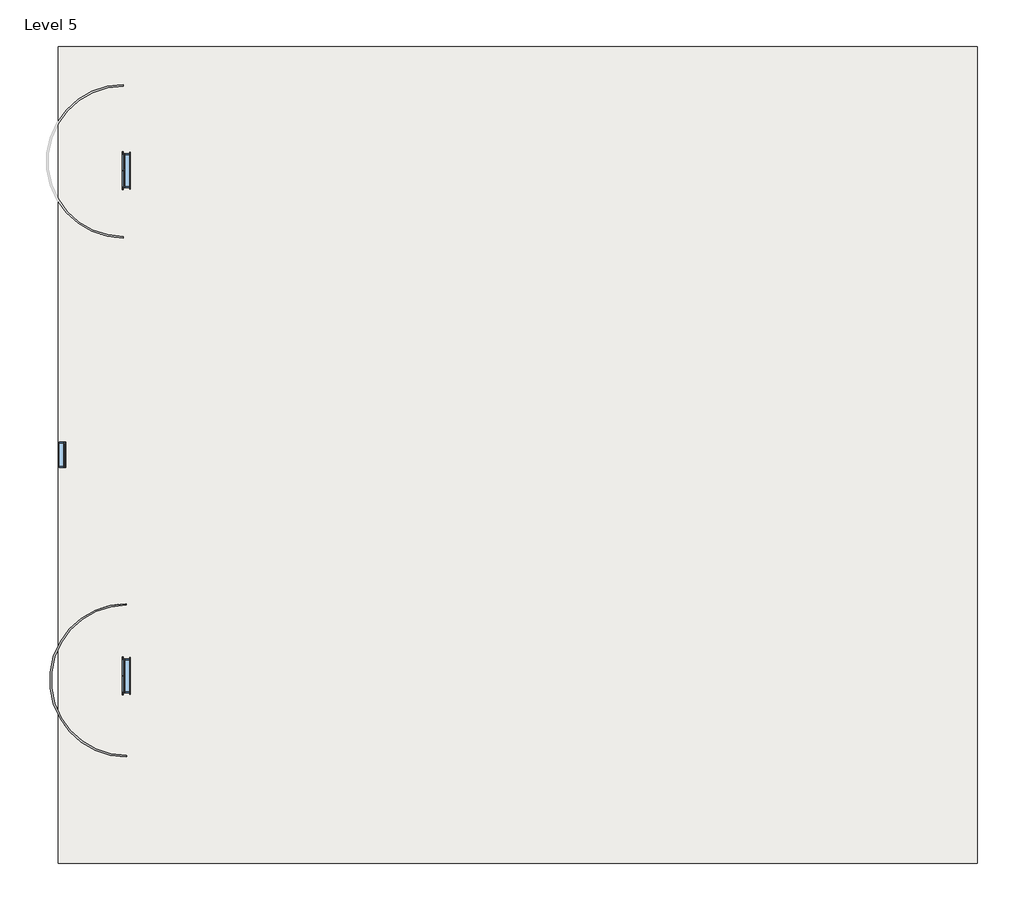
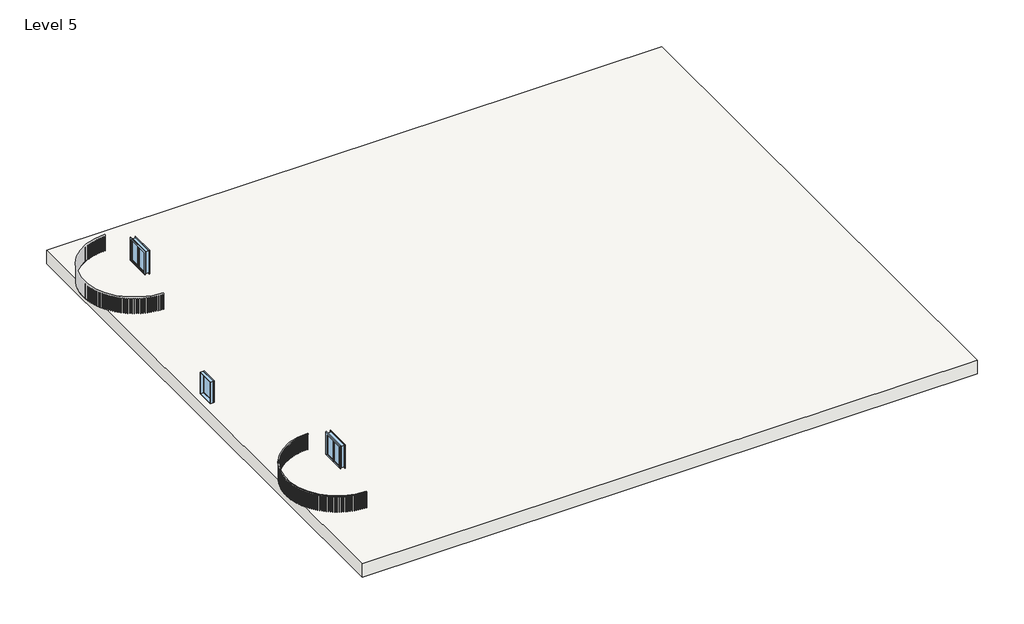
# One storey, part 1 of 2: 3 windows, 1 railing, 1 slab.
"""IFC4 building model written with IfcOpenShell, lengths in millimetres."""

from ifc_helpers import new_model, si_unit, point, frame, frame_2d, origin, place, context, project, spatial, polyline, circle_curve, trimmed, segment, composite_curve, outline, extrude, transform, mapped, element, save
from components import window_534dcd48, window_c1f32544

model = new_model("IFC4")

# Units and contexts
model_context = context("Model", 3, world=origin())
ifc_project = project(units=[si_unit("LENGTHUNIT", "METRE", prefix="MILLI")], contexts=[model_context])

# Site, building, storey
site = spatial("IfcSite", under=ifc_project)
building = spatial("IfcBuilding", under=site)
storey = spatial("IfcBuildingStorey", under=building, Name="Level 5", Elevation=12192.0)

# Railing
placement = place(None, origin())
element("IfcRailing", 1, ObjectType="Handrail - Rectangular", at=placement, inside=storey, context=model_context, shape_type="SweptSolid", body=[
    extrude(outline(composite_curve([segment(trimmed(circle_curve(frame_2d((-15613.8723021, -8267.0443987)), 2743.2), [point((-15613.8723021, -11010.2443987))], [point((-15613.8723021, -5523.8443987))], False, "CARTESIAN"), True, "CONTINUOUS"), segment(polyline([(-15613.8723021, -5523.8443987), (-15613.8723021, -5574.6443987)]), True, "CONTINUOUS"), segment(trimmed(circle_curve(frame_2d((-15613.8723021, -8267.0443987)), 2692.4), [point((-15613.8723021, -5574.6443987))], [point((-15613.8723021, -10959.4443987))], True, "CARTESIAN"), True, "CONTINUOUS"), segment(polyline([(-15613.8723021, -10959.4443987), (-15613.8723021, -11010.2443987)]), True, "CONTINUOUS")], self_intersect=False)), frame((0.0, 0.0, 13055.6), z_axis=(0.0, 0.0, 1.0), x_axis=(1.0, 0.0, 0.0)), (0.0, 0.0, 1.0), 50.8),
    extrude(outline(polyline([(-15627.231195, -10994.3533143), (-15627.2044157, -10975.3033331), (-15608.1544345, -10975.3301124), (-15608.1812138, -10994.3800936), (-15627.231195, -10994.3533143)])), frame((0.0, 0.0, 12192.0), z_axis=(0.0, 0.0, 1.0), x_axis=(1.0, 0.0, 0.0)), (0.0, 0.0, 1.0), 863.6),
    extrude(outline(polyline([(-15729.1535895, -10991.9485449), (-15728.414846, -10972.9128742), (-15709.3791753, -10973.6516178), (-15710.1179188, -10992.6872885), (-15729.1535895, -10991.9485449)])), frame((0.0, 0.0, 12192.0), z_axis=(0.0, 0.0, 1.0), x_axis=(1.0, 0.0, 0.0)), (0.0, 0.0, 1.0), 863.6),
    extrude(outline(polyline([(-15830.914897, -10985.7361601), (-15829.4652214, -10966.7413992), (-15810.4704606, -10968.1910747), (-15811.9201361, -10987.1858356), (-15830.914897, -10985.7361601)])), frame((0.0, 0.0, 12192.0), z_axis=(0.0, 0.0, 1.0), x_axis=(1.0, 0.0, 0.0)), (0.0, 0.0, 1.0), 863.6),
    extrude(outline(polyline([(-15932.3729223, -10975.7248406), (-15930.2143405, -10956.7975316), (-15911.2870315, -10958.9561134), (-15913.4456133, -10977.8834224), (-15932.3729223, -10975.7248406)])), frame((0.0, 0.0, 12192.0), z_axis=(0.0, 0.0, 1.0), x_axis=(1.0, 0.0, 0.0)), (0.0, 0.0, 1.0), 863.6),
    extrude(outline(polyline([(-16033.3858942, -10961.9285757), (-16030.5214224, -10943.0951665), (-16011.6880132, -10945.9596384), (-16014.5524851, -10964.7930475), (-16033.3858942, -10961.9285757)])), frame((0.0, 0.0, 12192.0), z_axis=(0.0, 0.0, 1.0), x_axis=(1.0, 0.0, 0.0)), (0.0, 0.0, 1.0), 863.6),
    extrude(outline(polyline([(-16133.8126634, -10944.3666434), (-16130.2463041, -10925.6534507), (-16111.5331114, -10929.2198099), (-16115.0994706, -10947.9330026), (-16133.8126634, -10944.3666434)])), frame((0.0, 0.0, 12192.0), z_axis=(0.0, 0.0, 1.0), x_axis=(1.0, 0.0, 0.0)), (0.0, 0.0, 1.0), 863.6),
    extrude(outline(polyline([(-16233.5128994, -10923.0635838), (-16229.2496362, -10904.4967562), (-16210.6828086, -10908.7600194), (-16214.9460718, -10927.326847), (-16233.5128994, -10923.0635838)])), frame((0.0, 0.0, 12192.0), z_axis=(0.0, 0.0, 1.0), x_axis=(1.0, 0.0, 0.0)), (0.0, 0.0, 1.0), 863.6),
    extrude(outline(polyline([(-16332.3472874, -10898.0491643), (-16327.3930774, -10879.654646), (-16308.9985591, -10884.608856), (-16313.9527691, -10903.0033743), (-16332.3472874, -10898.0491643)])), frame((0.0, 0.0, 12192.0), z_axis=(0.0, 0.0, 1.0), x_axis=(1.0, 0.0, 0.0)), (0.0, 0.0, 1.0), 863.6),
    extrude(outline(polyline([(-16430.1777221, -10869.3583388), (-16424.5394881, -10851.1618331), (-16406.3429824, -10856.8000671), (-16411.9812164, -10874.9965728), (-16430.1777221, -10869.3583388)])), frame((0.0, 0.0, 12192.0), z_axis=(0.0, 0.0, 1.0), x_axis=(1.0, 0.0, 0.0)), (0.0, 0.0, 1.0), 863.6),
    extrude(outline(polyline([(-16526.8675012, -10837.0311978), (-16520.5531216, -10819.0581316), (-16502.5800554, -10825.3725111), (-16508.8944349, -10843.3455773), (-16526.8675012, -10837.0311978)])), frame((0.0, 0.0, 12192.0), z_axis=(0.0, 0.0, 1.0), x_axis=(1.0, 0.0, 0.0)), (0.0, 0.0, 1.0), 863.6),
    extrude(outline(polyline([(-16622.2815163, -10801.1129136), (-16615.2998146, -10783.3884011), (-16597.5753021, -10790.3701028), (-16604.5570038, -10808.0946153), (-16622.2815163, -10801.1129136)])), frame((0.0, 0.0, 12192.0), z_axis=(0.0, 0.0, 1.0), x_axis=(1.0, 0.0, 0.0)), (0.0, 0.0, 1.0), 863.6),
    extrude(outline(polyline([(-16716.2864416, -10761.653676), (-16708.6471735, -10744.2024845), (-16691.1959821, -10751.8417526), (-16698.8352501, -10769.292944), (-16716.2864416, -10761.653676)])), frame((0.0, 0.0, 12192.0), z_axis=(0.0, 0.0, 1.0), x_axis=(1.0, 0.0, 0.0)), (0.0, 0.0, 1.0), 863.6),
    extrude(outline(polyline([(-16808.7509204, -10718.708623), (-16800.4647607, -10701.5551378), (-16783.3112754, -10709.8412975), (-16791.5974352, -10726.9947828), (-16808.7509204, -10718.708623)])), frame((0.0, 0.0, 12192.0), z_axis=(0.0, 0.0, 1.0), x_axis=(1.0, 0.0, 0.0)), (0.0, 0.0, 1.0), 863.6),
    extrude(outline(polyline([(-16899.5457485, -10672.3377634), (-16890.6242756, -10655.5059536), (-16873.7924658, -10664.4274266), (-16882.7139387, -10681.2592364), (-16899.5457485, -10672.3377634)])), frame((0.0, 0.0, 12192.0), z_axis=(0.0, 0.0, 1.0), x_axis=(1.0, 0.0, 0.0)), (0.0, 0.0, 1.0), 863.6),
    extrude(outline(polyline([(-16988.5440547, -10622.6058931), (-16978.9997349, -10606.1192785), (-16962.5131203, -10615.6635983), (-16972.0574401, -10632.1502129), (-16988.5440547, -10622.6058931)])), frame((0.0, 0.0, 12192.0), z_axis=(0.0, 0.0, 1.0), x_axis=(1.0, 0.0, 0.0)), (0.0, 0.0, 1.0), 863.6),
    extrude(outline(polyline([(-17075.621478, -10569.5825043), (-17065.4676481, -10553.4641223), (-17049.3492661, -10563.6179523), (-17059.5030961, -10579.7363343), (-17075.621478, -10569.5825043)])), frame((0.0, 0.0, 12192.0), z_axis=(0.0, 0.0, 1.0), x_axis=(1.0, 0.0, 0.0)), (0.0, 0.0, 1.0), 863.6),
    extrude(outline(polyline([(-17160.656342, -10513.3416887), (-17149.9071902, -10497.6140622), (-17134.1795637, -10508.363214), (-17144.9287154, -10524.0908405), (-17160.656342, -10513.3416887)])), frame((0.0, 0.0, 12192.0), z_axis=(0.0, 0.0, 1.0), x_axis=(1.0, 0.0, 0.0)), (0.0, 0.0, 1.0), 863.6),
    extrude(outline(polyline([(-17243.5298239, -10453.9620338), (-17232.2003705, -10438.6471396), (-17216.8854763, -10449.976593), (-17228.2149296, -10465.2914872), (-17243.5298239, -10453.9620338)])), frame((0.0, 0.0, 12192.0), z_axis=(0.0, 0.0, 1.0), x_axis=(1.0, 0.0, 0.0)), (0.0, 0.0, 1.0), 863.6),
    extrude(outline(polyline([(-17324.1261214, -10391.5265132), (-17312.2321975, -10376.6457513), (-17297.3514357, -10388.5396752), (-17309.2453596, -10403.4204371), (-17324.1261214, -10391.5265132)])), frame((0.0, 0.0, 12192.0), z_axis=(0.0, 0.0, 1.0), x_axis=(1.0, 0.0, 0.0)), (0.0, 0.0, 1.0), 863.6),
    extrude(outline(polyline([(-17402.3326143, -10326.1223703), (-17389.8908397, -10311.6965343), (-17375.4650036, -10324.1383088), (-17387.9067782, -10338.5641449), (-17402.3326143, -10326.1223703)])), frame((0.0, 0.0, 12192.0), z_axis=(0.0, 0.0, 1.0), x_axis=(1.0, 0.0, 0.0)), (0.0, 0.0, 1.0), 863.6),
    extrude(outline(polyline([(-17478.0400213, -10257.840997), (-17465.0677814, -10243.8902446), (-17451.117029, -10256.8624845), (-17464.0892689, -10270.8132369), (-17478.0400213, -10257.840997)])), frame((0.0, 0.0, 12192.0), z_axis=(0.0, 0.0, 1.0), x_axis=(1.0, 0.0, 0.0)), (0.0, 0.0, 1.0), 863.6),
    extrude(outline(polyline([(-17551.1425537, -10186.7778056), (-17537.6579752, -10173.3216307), (-17524.2018003, -10186.8062093), (-17537.6863789, -10200.2623841), (-17551.1425537, -10186.7778056)])), frame((0.0, 0.0, 12192.0), z_axis=(0.0, 0.0, 1.0), x_axis=(1.0, 0.0, 0.0)), (0.0, 0.0, 1.0), 863.6),
    extrude(outline(polyline([(-17621.5380624, -10113.0320953), (-17607.5599877, -10100.0893009), (-17594.6171933, -10114.0673756), (-17608.595268, -10127.01017), (-17621.5380624, -10113.0320953)])), frame((0.0, 0.0, 12192.0), z_axis=(0.0, 0.0, 1.0), x_axis=(1.0, 0.0, 0.0)), (0.0, 0.0, 1.0), 863.6),
    extrude(outline(polyline([(-17689.128181, -10036.7069141), (-17674.6761422, -10024.2955856), (-17662.2648137, -10038.7476243), (-17676.7168525, -10051.1589528), (-17689.128181, -10036.7069141)])), frame((0.0, 0.0, 12192.0), z_axis=(0.0, 0.0, 1.0), x_axis=(1.0, 0.0, 0.0)), (0.0, 0.0, 1.0), 863.6),
    extrude(outline(polyline([(-17753.8184631, -9957.908914), (-17738.9126547, -9946.0463942), (-17727.0501349, -9960.9522026), (-17741.9559433, -9972.8147224), (-17753.8184631, -9957.908914)])), frame((0.0, 0.0, 12192.0), z_axis=(0.0, 0.0, 1.0), x_axis=(1.0, 0.0, 0.0)), (0.0, 0.0, 1.0), 863.6),
    extrude(outline(polyline([(-17815.5185146, -9876.7482026), (-17800.179765, -9865.4510675), (-17788.8826299, -9880.789817), (-17804.2213795, -9892.0869522), (-17815.5185146, -9876.7482026)])), frame((0.0, 0.0, 12192.0), z_axis=(0.0, 0.0, 1.0), x_axis=(1.0, 0.0, 0.0)), (0.0, 0.0, 1.0), 863.6),
    extrude(outline(polyline([(-17874.1421194, -9793.338189), (-17858.3918621, -9782.6222244), (-17847.6758976, -9798.3724817), (-17863.4261549, -9809.0884462), (-17874.1421194, -9793.338189)])), frame((0.0, 0.0, 12192.0), z_axis=(0.0, 0.0, 1.0), x_axis=(1.0, 0.0, 0.0)), (0.0, 0.0, 1.0), 863.6),
    extrude(outline(polyline([(-17929.6073606, -9707.7954251), (-17913.467604, -9697.6756051), (-17903.347784, -9713.8153616), (-17919.4875405, -9723.9351817), (-17929.6073606, -9707.7954251)])), frame((0.0, 0.0, 12192.0), z_axis=(0.0, 0.0, 1.0), x_axis=(1.0, 0.0, 0.0)), (0.0, 0.0, 1.0), 863.6),
    extrude(outline(polyline([(-17981.8367343, -9620.2394434), (-17965.3300312, -9610.7299086), (-17955.8204964, -9627.2366117), (-17972.3271995, -9636.7461465), (-17981.8367343, -9620.2394434)])), frame((0.0, 0.0, 12192.0), z_axis=(0.0, 0.0, 1.0), x_axis=(1.0, 0.0, 0.0)), (0.0, 0.0, 1.0), 863.6),
    extrude(outline(polyline([(-18030.7572585, -9530.7925891), (-18013.9066743, -9521.9066277), (-18005.0207128, -9538.7572119), (-18021.871297, -9547.6431733), (-18030.7572585, -9530.7925891)])), frame((0.0, 0.0, 12192.0), z_axis=(0.0, 0.0, 1.0), x_axis=(1.0, 0.0, 0.0)), (0.0, 0.0, 1.0), 863.6),
    extrude(outline(polyline([(-18076.3005745, -9439.5798499), (-18059.1296552, -9431.3298785), (-18050.8796837, -9448.5007978), (-18068.0506031, -9456.7507693), (-18076.3005745, -9439.5798499)])), frame((0.0, 0.0, 12192.0), z_axis=(0.0, 0.0, 1.0), x_axis=(1.0, 0.0, 0.0)), (0.0, 0.0, 1.0), 863.6),
    extrude(outline(polyline([(-18118.4030429, -9346.728681), (-18100.9357821, -9339.1262276), (-18093.3333287, -9356.5934885), (-18110.8005895, -9364.1959419), (-18118.4030429, -9346.728681)])), frame((0.0, 0.0, 12192.0), z_axis=(0.0, 0.0, 1.0), x_axis=(1.0, 0.0, 0.0)), (0.0, 0.0, 1.0), 863.6),
    extrude(outline(polyline([(-18157.0058323, -9252.3688268), (-18139.2666376, -9245.4245147), (-18132.3223254, -9263.1637094), (-18150.0615201, -9270.1080215), (-18157.0058323, -9252.3688268)])), frame((0.0, 0.0, 12192.0), z_axis=(0.0, 0.0, 1.0), x_axis=(1.0, 0.0, 0.0)), (0.0, 0.0, 1.0), 863.6),
    extrude(outline(polyline([(-18192.0550015, -9156.6321402), (-18174.0686606, -9150.3556729), (-18167.7921932, -9168.3420137), (-18185.7785341, -9174.6184811), (-18192.0550015, -9156.6321402)])), frame((0.0, 0.0, 12192.0), z_axis=(0.0, 0.0, 1.0), x_axis=(1.0, 0.0, 0.0)), (0.0, 0.0, 1.0), 863.6),
    extrude(outline(polyline([(-18223.5015748, -9059.6523978), (-18205.2932208, -9054.0525456), (-18199.6933686, -9072.2608996), (-18217.9017226, -9077.8607518), (-18223.5015748, -9059.6523978)])), frame((0.0, 0.0, 12192.0), z_axis=(0.0, 0.0, 1.0), x_axis=(1.0, 0.0, 0.0)), (0.0, 0.0, 1.0), 863.6),
    extrude(outline(polyline([(-18251.3016108, -8961.5651131), (-18232.8966869, -8956.6497009), (-18227.9812748, -8975.0546248), (-18246.3861986, -8979.970037), (-18251.3016108, -8961.5651131)])), frame((0.0, 0.0, 12192.0), z_axis=(0.0, 0.0, 1.0), x_axis=(1.0, 0.0, 0.0)), (0.0, 0.0, 1.0), 863.6),
    extrude(outline(polyline([(-18275.4162634, -8862.5073473), (-18256.8404876, -8858.2832437), (-18252.6163839, -8876.8590196), (-18271.1921598, -8881.0831232), (-18275.4162634, -8862.5073473)])), frame((0.0, 0.0, 12192.0), z_axis=(0.0, 0.0, 1.0), x_axis=(1.0, 0.0, 0.0)), (0.0, 0.0, 1.0), 863.6),
    extrude(outline(polyline([(-18295.8118362, -8762.6175179), (-18277.0911651, -8759.0906253), (-18273.5642725, -8777.8112965), (-18292.2849436, -8781.338189), (-18295.8118362, -8762.6175179)])), frame((0.0, 0.0, 12192.0), z_axis=(0.0, 0.0, 1.0), x_axis=(1.0, 0.0, 0.0)), (0.0, 0.0, 1.0), 863.6),
    extrude(outline(polyline([(-18312.4598298, -8662.0352047), (-18293.6204224, -8659.2104514), (-18290.7956691, -8678.0498587), (-18309.6350765, -8680.874612), (-18312.4598298, -8662.0352047)])), frame((0.0, 0.0, 12192.0), z_axis=(0.0, 0.0, 1.0), x_axis=(1.0, 0.0, 0.0)), (0.0, 0.0, 1.0), 863.6),
    extrude(outline(polyline([(-18325.3369811, -8560.9009553), (-18306.4051626, -8558.7822885), (-18304.2864958, -8577.714107), (-18323.2183143, -8579.8327738), (-18325.3369811, -8560.9009553)])), frame((0.0, 0.0, 12192.0), z_axis=(0.0, 0.0, 1.0), x_axis=(1.0, 0.0, 0.0)), (0.0, 0.0, 1.0), 863.6),
    extrude(outline(polyline([(-18334.4252965, -8459.3560886), (-18315.427521, -8457.9464688), (-18314.0179011, -8476.9442442), (-18333.0156766, -8478.3538641), (-18334.4252965, -8459.3560886)])), frame((0.0, 0.0, 12192.0), z_axis=(0.0, 0.0, 1.0), x_axis=(1.0, 0.0, 0.0)), (0.0, 0.0, 1.0), 863.6),
    extrude(outline(polyline([(-18339.7120764, -8357.5424973), (-18320.6748904, -8356.8438941), (-18319.9762872, -8375.8810802), (-18339.0134732, -8376.5796834), (-18339.7120764, -8357.5424973)])), frame((0.0, 0.0, 12192.0), z_axis=(0.0, 0.0, 1.0), x_axis=(1.0, 0.0, 0.0)), (0.0, 0.0, 1.0), 863.6),
    extrude(outline(polyline([(-18341.1899336, -8255.6024494), (-18322.1399383, -8255.6158391), (-18322.1533279, -8274.6658344), (-18341.2033232, -8274.6524447), (-18341.1899336, -8255.6024494)])), frame((0.0, 0.0, 12192.0), z_axis=(0.0, 0.0, 1.0), x_axis=(1.0, 0.0, 0.0)), (0.0, 0.0, 1.0), 863.6),
    extrude(outline(polyline([(-18338.8568028, -8153.6783898), (-18319.8206176, -8154.4037536), (-18320.5459814, -8173.4399388), (-18339.5821666, -8172.7145751), (-18338.8568028, -8153.6783898)])), frame((0.0, 0.0, 12192.0), z_axis=(0.0, 0.0, 1.0), x_axis=(1.0, 0.0, 0.0)), (0.0, 0.0, 1.0), 863.6),
    extrude(outline(polyline([(-18332.7159444, -8051.912741), (-18313.7201692, -8053.3490654), (-18315.1564936, -8072.3448405), (-18334.1522687, -8070.9085161), (-18332.7159444, -8051.912741)])), frame((0.0, 0.0, 12192.0), z_axis=(0.0, 0.0, 1.0), x_axis=(1.0, 0.0, 0.0)), (0.0, 0.0, 1.0), 863.6),
    extrude(outline(polyline([(-18322.775939, -7950.4477041), (-18303.8471175, -7952.592982), (-18305.9923954, -7971.5218035), (-18324.9212169, -7969.3765256), (-18322.775939, -7950.4477041)])), frame((0.0, 0.0, 12192.0), z_axis=(0.0, 0.0, 1.0), x_axis=(1.0, 0.0, 0.0)), (0.0, 0.0, 1.0), 863.6),
    extrude(outline(polyline([(-18309.0506764, -7849.4250602), (-18290.2152585, -7852.2762939), (-18293.0664923, -7871.1117118), (-18311.9019101, -7868.260478), (-18309.0506764, -7849.4250602)])), frame((0.0, 0.0, 12192.0), z_axis=(0.0, 0.0, 1.0), x_axis=(1.0, 0.0, 0.0)), (0.0, 0.0, 1.0), 863.6),
    extrude(outline(polyline([(-18291.5593353, -7748.9859721), (-18272.8436405, -7752.5391776), (-18276.396846, -7771.2548723), (-18295.1125408, -7767.7016669), (-18291.5593353, -7748.9859721)])), frame((0.0, 0.0, 12192.0), z_axis=(0.0, 0.0, 1.0), x_axis=(1.0, 0.0, 0.0)), (0.0, 0.0, 1.0), 863.6),
    extrude(outline(polyline([(-18270.3263571, -7649.2707874), (-18251.7565376, -7653.5209995), (-18256.0067497, -7672.0908191), (-18274.5765692, -7667.8406069), (-18270.3263571, -7649.2707874)])), frame((0.0, 0.0, 12192.0), z_axis=(0.0, 0.0, 1.0), x_axis=(1.0, 0.0, 0.0)), (0.0, 0.0, 1.0), 863.6),
    extrude(outline(polyline([(-18245.3814115, -7550.418842), (-18226.9834156, -7555.3601218), (-18231.9246954, -7573.7581178), (-18250.3226913, -7568.816838), (-18245.3814115, -7550.418842)])), frame((0.0, 0.0, 12192.0), z_axis=(0.0, 0.0, 1.0), x_axis=(1.0, 0.0, 0.0)), (0.0, 0.0, 1.0), 863.6),
    extrude(outline(polyline([(-18216.7593549, -7452.5682656), (-18198.5588909, -7458.1937085), (-18204.1843337, -7476.3941726), (-18222.3847978, -7470.7687297), (-18216.7593549, -7452.5682656)])), frame((0.0, 0.0, 12192.0), z_axis=(0.0, 0.0, 1.0), x_axis=(1.0, 0.0, 0.0)), (0.0, 0.0, 1.0), 863.6),
    extrude(outline(polyline([(-18184.5001822, -7355.8557887), (-18166.5226822, -7362.1575339), (-18172.8244275, -7380.1350339), (-18190.8019275, -7373.8332887), (-18184.5001822, -7355.8557887)])), frame((0.0, 0.0, 12192.0), z_axis=(0.0, 0.0, 1.0), x_axis=(1.0, 0.0, 0.0)), (0.0, 0.0, 1.0), 863.6),
    extrude(outline(polyline([(-18148.6489704, -7260.4165513), (-18130.9195551, -7267.3857933), (-18137.888797, -7285.1152086), (-18155.6182123, -7278.1459666), (-18148.6489704, -7260.4165513)])), frame((0.0, 0.0, 12192.0), z_axis=(0.0, 0.0, 1.0), x_axis=(1.0, 0.0, 0.0)), (0.0, 0.0, 1.0), 863.6),
    extrude(outline(polyline([(-18109.2558157, -7166.3839145), (-18091.7992591, -7174.0109148), (-18099.4262594, -7191.4674713), (-18116.8828159, -7183.8404711), (-18109.2558157, -7166.3839145)])), frame((0.0, 0.0, 12192.0), z_axis=(0.0, 0.0, 1.0), x_axis=(1.0, 0.0, 0.0)), (0.0, 0.0, 1.0), 863.6),
    extrude(outline(polyline([(-18066.3757637, -7073.8892738), (-18049.2164586, -7082.1633749), (-18057.4905597, -7099.32268), (-18074.6498648, -7091.0485789), (-18066.3757637, -7073.8892738)])), frame((0.0, 0.0, 12192.0), z_axis=(0.0, 0.0, 1.0), x_axis=(1.0, 0.0, 0.0)), (0.0, 0.0, 1.0), 863.6),
    extrude(outline(polyline([(-18020.0687324, -6983.0618755), (-18003.2306562, -6991.9715157), (-18012.1402963, -7008.8095919), (-18028.9783726, -6999.8999518), (-18020.0687324, -6983.0618755)])), frame((0.0, 0.0, 12192.0), z_axis=(0.0, 0.0, 1.0), x_axis=(1.0, 0.0, 0.0)), (0.0, 0.0, 1.0), 863.6),
    extrude(outline(polyline([(-17970.3994285, -6894.0286364), (-17953.9061096, -6903.5613658), (-17963.4388391, -6920.0546848), (-17979.932158, -6910.5219553), (-17970.3994285, -6894.0286364)])), frame((0.0, 0.0, 12192.0), z_axis=(0.0, 0.0, 1.0), x_axis=(1.0, 0.0, 0.0)), (0.0, 0.0, 1.0), 863.6),
    extrude(outline(polyline([(-17917.4372568, -6806.913966), (-17901.311742, -6817.0564643), (-17911.4542403, -6833.1819791), (-17927.5797552, -6823.0394808), (-17917.4372568, -6806.913966)])), frame((0.0, 0.0, 12192.0), z_axis=(0.0, 0.0, 1.0), x_axis=(1.0, 0.0, 0.0)), (0.0, 0.0, 1.0), 863.6),
    extrude(outline(polyline([(-17861.2562235, -6721.8395932), (-17845.5210456, -6732.5776878), (-17856.2591402, -6748.3128657), (-17871.9943181, -6737.5747711), (-17861.2562235, -6721.8395932)])), frame((0.0, 0.0, 12192.0), z_axis=(0.0, 0.0, 1.0), x_axis=(1.0, 0.0, 0.0)), (0.0, 0.0, 1.0), 863.6),
    extrude(outline(polyline([(-17801.9348324, -6638.9243956), (-17786.6119788, -6650.2430818), (-17797.9306651, -6665.5659354), (-17813.2535187, -6654.2472492), (-17801.9348324, -6638.9243956)])), frame((0.0, 0.0, 12192.0), z_axis=(0.0, 0.0, 1.0), x_axis=(1.0, 0.0, 0.0)), (0.0, 0.0, 1.0), 863.6),
    extrude(outline(polyline([(-17739.5559758, -6558.284234), (-17724.6668577, -6570.1676957), (-17736.5503195, -6585.0568138), (-17751.4394375, -6573.1733521), (-17739.5559758, -6558.284234)])), frame((0.0, 0.0, 12192.0), z_axis=(0.0, 0.0, 1.0), x_axis=(1.0, 0.0, 0.0)), (0.0, 0.0, 1.0), 863.6),
    extrude(outline(polyline([(-17674.206818, -6480.03179), (-17659.7722406, -6492.463422), (-17672.2038726, -6506.8979994), (-17686.63845, -6494.4663674), (-17674.206818, -6480.03179)])), frame((0.0, 0.0, 12192.0), z_axis=(0.0, 0.0, 1.0), x_axis=(1.0, 0.0, 0.0)), (0.0, 0.0, 1.0), 863.6),
    extrude(outline(polyline([(-17605.978674, -6404.2764087), (-17592.0188072, -6417.2388399), (-17604.9812384, -6431.1987066), (-17618.9411051, -6418.2362755), (-17605.978674, -6404.2764087)])), frame((0.0, 0.0, 12192.0), z_axis=(0.0, 0.0, 1.0), x_axis=(1.0, 0.0, 0.0)), (0.0, 0.0, 1.0), 863.6),
    extrude(outline(polyline([(-17534.9668816, -6331.1239463), (-17521.5012322, -6344.5990636), (-17534.9763495, -6358.064713), (-17548.4419989, -6344.5895957), (-17534.9668816, -6331.1239463)])), frame((0.0, 0.0, 12192.0), z_axis=(0.0, 0.0, 1.0), x_axis=(1.0, 0.0, 0.0)), (0.0, 0.0, 1.0), 863.6),
    extrude(outline(polyline([(-17461.2706683, -6260.6766214), (-17448.3180524, -6274.6455956), (-17462.2870265, -6287.5982116), (-17475.2396425, -6273.6292374), (-17461.2706683, -6260.6766214)])), frame((0.0, 0.0, 12192.0), z_axis=(0.0, 0.0, 1.0), x_axis=(1.0, 0.0, 0.0)), (0.0, 0.0, 1.0), 863.6),
    extrude(outline(polyline([(-17384.9930129, -6193.032873), (-17372.5715296, -6207.4761846), (-17387.0148412, -6219.897668), (-17399.4363246, -6205.4543563), (-17384.9930129, -6193.032873)])), frame((0.0, 0.0, 12192.0), z_axis=(0.0, 0.0, 1.0), x_axis=(1.0, 0.0, 0.0)), (0.0, 0.0, 1.0), 863.6),
    extrude(outline(polyline([(-17306.2405011, -6128.2872222), (-17294.3675074, -6143.1846891), (-17309.2649743, -6155.0576828), (-17321.137968, -6140.1602159), (-17306.2405011, -6128.2872222)])), frame((0.0, 0.0, 12192.0), z_axis=(0.0, 0.0, 1.0), x_axis=(1.0, 0.0, 0.0)), (0.0, 0.0, 1.0), 863.6),
    extrude(outline(polyline([(-17225.1231768, -6066.5301406), (-17213.8152633, -6081.860946), (-17229.1460687, -6093.1688594), (-17240.4539822, -6077.8380541), (-17225.1231768, -6066.5301406)])), frame((0.0, 0.0, 12192.0), z_axis=(0.0, 0.0, 1.0), x_axis=(1.0, 0.0, 0.0)), (0.0, 0.0, 1.0), 863.6),
    extrude(outline(polyline([(-17141.7543884, -6007.847924), (-17131.0273562, -6023.5906455), (-17146.7700777, -6034.3176777), (-17157.4971099, -6018.5749562), (-17141.7543884, -6007.847924)])), frame((0.0, 0.0, 12192.0), z_axis=(0.0, 0.0, 1.0), x_axis=(1.0, 0.0, 0.0)), (0.0, 0.0, 1.0), 863.6),
    extrude(outline(polyline([(-17056.2506305, -5952.3225712), (-17046.1194688, -5968.4552108), (-17062.2521085, -5978.5863725), (-17072.3832702, -5962.4537328), (-17056.2506305, -5952.3225712)])), frame((0.0, 0.0, 12192.0), z_axis=(0.0, 0.0, 1.0), x_axis=(1.0, 0.0, 0.0)), (0.0, 0.0, 1.0), 863.6),
    extrude(outline(polyline([(-16968.7313808, -5900.03167), (-16959.2102463, -5916.5316851), (-16975.7102614, -5926.0528195), (-16985.2313959, -5909.5528044), (-16968.7313808, -5900.03167)])), frame((0.0, 0.0, 12192.0), z_axis=(0.0, 0.0, 1.0), x_axis=(1.0, 0.0, 0.0)), (0.0, 0.0, 1.0), 863.6),
    extrude(outline(polyline([(-16879.3189333, -5851.0482885), (-16870.4211303, -5867.8926229), (-16887.2654647, -5876.7904259), (-16896.1632677, -5859.9460915), (-16879.3189333, -5851.0482885)])), frame((0.0, 0.0, 12192.0), z_axis=(0.0, 0.0, 1.0), x_axis=(1.0, 0.0, 0.0)), (0.0, 0.0, 1.0), 863.6),
    extrude(outline(polyline([(-16788.1382277, -5805.4408731), (-16779.8761894, -5822.6059896), (-16797.0413058, -5830.8680279), (-16805.3033441, -5813.7029114), (-16788.1382277, -5805.4408731)])), frame((0.0, 0.0, 12192.0), z_axis=(0.0, 0.0, 1.0), x_axis=(1.0, 0.0, 0.0)), (0.0, 0.0, 1.0), 863.6),
    extrude(outline(polyline([(-16695.3166742, -5763.2731529), (-16687.7019455, -5780.7350659), (-16705.1638585, -5788.3497946), (-16712.7785872, -5770.8878816), (-16695.3166742, -5763.2731529)])), frame((0.0, 0.0, 12192.0), z_axis=(0.0, 0.0, 1.0), x_axis=(1.0, 0.0, 0.0)), (0.0, 0.0, 1.0), 863.6),
    extrude(outline(polyline([(-16600.983976, -5724.6040505), (-16594.0271973, -5742.3383598), (-16611.7615066, -5749.2951386), (-16618.7182854, -5731.5608292), (-16600.983976, -5724.6040505)])), frame((0.0, 0.0, 12192.0), z_axis=(0.0, 0.0, 1.0), x_axis=(1.0, 0.0, 0.0)), (0.0, 0.0, 1.0), 863.6),
    extrude(outline(polyline([(-16505.271948, -5689.4875996), (-16498.9828402, -5707.4695245), (-16516.9647651, -5713.7586324), (-16523.2538729, -5695.7767075), (-16505.271948, -5689.4875996)])), frame((0.0, 0.0, 12192.0), z_axis=(0.0, 0.0, 1.0), x_axis=(1.0, 0.0, 0.0)), (0.0, 0.0, 1.0), 863.6),
    extrude(outline(polyline([(-16408.3143324, -5657.97287), (-16402.7016834, -5676.1772836), (-16420.906097, -5681.7899325), (-16426.5187459, -5663.5855189), (-16408.3143324, -5657.97287)])), frame((0.0, 0.0, 12192.0), z_axis=(0.0, 0.0, 1.0), x_axis=(1.0, 0.0, 0.0)), (0.0, 0.0, 1.0), 863.6),
    extrude(outline(polyline([(-16310.2466117, -5630.1038984), (-16305.3182645, -5648.5053628), (-16323.7197289, -5653.43371), (-16328.6480761, -5635.0322456), (-16310.2466117, -5630.1038984)])), frame((0.0, 0.0, 12192.0), z_axis=(0.0, 0.0, 1.0), x_axis=(1.0, 0.0, 0.0)), (0.0, 0.0, 1.0), 863.6),
    extrude(outline(polyline([(-16211.2058198, -5605.9196271), (-16206.9686609, -5624.4924294), (-16225.5414632, -5628.7295883), (-16229.7786221, -5610.1567861), (-16211.2058198, -5605.9196271)])), frame((0.0, 0.0, 12192.0), z_axis=(0.0, 0.0, 1.0), x_axis=(1.0, 0.0, 0.0)), (0.0, 0.0, 1.0), 863.6),
    extrude(outline(polyline([(-16111.3303505, -5585.4538499), (-16107.7903006, -5604.1720375), (-16126.5084882, -5607.7120874), (-16130.048538, -5588.9938998), (-16111.3303505, -5585.4538499)])), frame((0.0, 0.0, 12192.0), z_axis=(0.0, 0.0, 1.0), x_axis=(1.0, 0.0, 0.0)), (0.0, 0.0, 1.0), 863.6),
    extrude(outline(polyline([(-16010.7597634, -5568.7351643), (-16007.9217692, -5587.5725816), (-16026.7591865, -5590.4105758), (-16029.5971807, -5571.5731585), (-16010.7597634, -5568.7351643)])), frame((0.0, 0.0, 12192.0), z_axis=(0.0, 0.0, 1.0), x_axis=(1.0, 0.0, 0.0)), (0.0, 0.0, 1.0), 863.6),
    extrude(outline(polyline([(-15909.63459, -5555.7869321), (-15907.5026171, -5574.7172567), (-15926.4329418, -5576.8492296), (-15928.5649146, -5557.918905), (-15909.63459, -5555.7869321)])), frame((0.0, 0.0, 12192.0), z_axis=(0.0, 0.0, 1.0), x_axis=(1.0, 0.0, 0.0)), (0.0, 0.0, 1.0), 863.6),
    extrude(outline(polyline([(-15808.0961363, -5546.6272462), (-15806.6731638, -5565.6240262), (-15825.6699438, -5567.0469987), (-15827.0929163, -5548.0502187), (-15808.0961363, -5546.6272462)])), frame((0.0, 0.0, 12192.0), z_axis=(0.0, 0.0, 1.0), x_axis=(1.0, 0.0, 0.0)), (0.0, 0.0, 1.0), 863.6),
    extrude(outline(polyline([(-15706.286286, -5541.268906), (-15705.5743024, -5560.3055963), (-15724.6109927, -5561.01758), (-15725.3229764, -5541.9808896), (-15706.286286, -5541.268906)])), frame((0.0, 0.0, 12192.0), z_axis=(0.0, 0.0, 1.0), x_axis=(1.0, 0.0, 0.0)), (0.0, 0.0, 1.0), 863.6),
    extrude(outline(polyline([(-15632.955606, -10994.3192673), (-15632.8888422, -10975.2693843), (-15613.8389591, -10975.3361482), (-15613.905723, -10994.3860312), (-15632.955606, -10994.3192673)])), frame((0.0, 0.0, 12192.0), z_axis=(0.0, 0.0, 1.0), x_axis=(1.0, 0.0, 0.0)), (0.0, 0.0, 1.0), 863.6),
    extrude(outline(polyline([(-15613.905723, -5539.7027662), (-15613.8389591, -5558.7526493), (-15632.8888422, -5558.8194131), (-15632.955606, -5539.7695301), (-15613.905723, -5539.7027662)])), frame((0.0, 0.0, 12192.0), z_axis=(0.0, 0.0, 1.0), x_axis=(1.0, 0.0, 0.0)), (0.0, 0.0, 1.0), 863.6),
])

# Slab
element("IfcSlab", 2, ObjectType="Generic - 12\"", at=placement, inside=storey, context=model_context, shape_type="SweptSolid", body=[
    extrude(outline(polyline([(14866.1276979, 14440.5556013), (14866.1276979, -14820.2443987), (-18052.2723021, -14820.2443987), (-18052.2723021, 14440.5556013), (14866.1276979, 14440.5556013)])), frame((0.0, 0.0, 11430.0), z_axis=(0.0, 0.0, 1.0), x_axis=(1.0, 0.0, 0.0)), (0.0, 0.0, 1.0), 762.0),
])

# Windows
window_shape = window_534dcd48(model_context)
element("IfcWindow", 3, ObjectType="Casement Dbl with Trim : 48\" x 48\"", at=placement, inside=storey, context=model_context, shape_type="MappedRepresentation", body=[
    mapped(window_shape, transform((-15594.8223021, 9995.5556013, 12192.0), x_axis=(0.0, 1.0, 0.0), y_axis=(-1.0, 0.0, 0.0), z_axis=(0.0, 0.0, 1.0))),
])
element("IfcWindow", 4, ObjectType="Casement Dbl with Trim : 48\" x 48\"", at=placement, inside=storey, context=model_context, shape_type="MappedRepresentation", body=[
    mapped(window_shape, transform((-15594.8223021, -8114.6443987, 12192.0), x_axis=(0.0, 1.0, 0.0), y_axis=(-1.0, 0.0, 0.0), z_axis=(0.0, 0.0, 1.0))),
])
window_2_shape = window_c1f32544(model_context)
element("IfcWindow", 5, ObjectType="Fixed : 36\" x 48\"", at=placement, inside=storey, context=model_context, shape_type="MappedRepresentation", body=[
    mapped(window_2_shape, transform((-17899.8723021, -227.9443987, 11735.1091362), x_axis=(0.0, -1.0, 0.0), y_axis=(1.0, 0.0, 0.0), z_axis=(0.0, 0.0, 1.0))),
])

save(model, "model.ifc")

# Revit data of these elements
# Type "Handrail - Rectangular"
#   Assembly Code = "C2010400"
#   built-in parameter 1008612 = 0.0416667 (stored number, unit not read)
#   built-in parameter 1008611 = 0.0416667 (stored number, unit not read)
#   built-in parameter 1008609 = 0.333333 (stored number, unit not read)
#   built-in parameter 1008604 = 0.166667 (stored number, unit not read)
#   built-in parameter 1008603 = 0.166667 (stored number, unit not read)
#   Railing Height = 3' - 0"
#   built-in parameter 1008630 = 2
#   built-in parameter 1008610 = 2
#   built-in parameter 1008618 = Baluster - Square : 3/4"
# Type "Generic - 12\""
#   Assembly Code = "B1010"
#   Function = 0
#   Layers, outside or top first: 2' - 6" no material (function 1)
# Type "Casement Dbl with Trim : 48\" x 48\""
#   Type Mark = "19"
#   Construction Type Id = "GSP4R"
#   Assembly Code = "B2020100"
#   Analytic Construction = "1/8 in Pilkington single glazing"
#   Visual Light Transmittance = 0.9
#   Solar Heat Gain Coefficient = 0.78
#   Heat Transfer Coefficient (U) = 0.6496 BTU/(h·ft²·°F)
#   Height = 4' - 0"
#   Default Sill Height = 3' - 0"
#   Trim Projection - Ext. = 0' - 0 1/2"
#   Trim Projection - Int. = 0' - 0 3/4"
#   Trim Width - Exterior = 0' - 3 1/2"
#   Trim Width - Interior = 0' - 3 1/2"
#   Width = 4' - 0"
#   Window Inset = 0' - 0 3/4"
#   Define Thermal Properties by = 1
#   Glass Pane Material = Glass
#   Sash Material = Sash
#   Trim Exterior Material = Trim
#   Trim Interior Material = Trim
#   Wall Closure = (empty or 0)
# Type "Fixed : 36\" x 48\""
#   Type Mark = "1"
#   Construction Type Id = "GSP4R"
#   Assembly Code = "B2020100"
#   Analytic Construction = "1/8 in Pilkington single glazing"
#   Visual Light Transmittance = 0.9
#   Solar Heat Gain Coefficient = 0.78
#   Heat Transfer Coefficient (U) = 0.6496 BTU/(h·ft²·°F)
#   Height = 4' - 0"
#   Default Sill Height = 3' - 0"
#   Width = 3' - 0"
#   Window Inset = 0' - 0 3/4"
#   Define Thermal Properties by = 1
#   Glass Pane Material = Glass
#   Sash Material = Sash
#   Wall Closure = (empty or 0)
# Element 1 (IfcRailing, "Handrail - Rectangular")
#   Phase Created = New Construction
# Element 2 (IfcSlab, "Generic - 12\"")
#   Height Offset From Level = 0' - 0"
#   Phase Created = New Construction
#   Materials on its faces: "Default Floor"
# Element 3 (IfcWindow, "Casement Dbl with Trim : 48\" x 48\"")
#   Mark = "9"
#   Phase Created = New Construction
#   Materials on its faces: "Sash", "Trim", "Glass"
# Element 4 (IfcWindow, "Casement Dbl with Trim : 48\" x 48\"")
#   Mark = "12"
#   Phase Created = New Construction
#   Materials on its faces: "Sash", "Trim", "Glass"
# Element 5 (IfcWindow, "Fixed : 36\" x 48\"")
#   Mark = "20"
#   Phase Created = New Construction
#   Materials on its faces: "Sash", "Glass"
# Materials
#   "Glass": class "Glass", colour RGB 0 128 192, transparency 0.75, Description = "Soda Lime Glass", Cost = 0
#   "Sash": class "Wood", colour RGB 224 178 126, transparency 0
#   "Trim": class "Wood", colour RGB 224 178 126, transparency 0
#   "Default Floor": colour RGB 128 128 128, transparency 0
